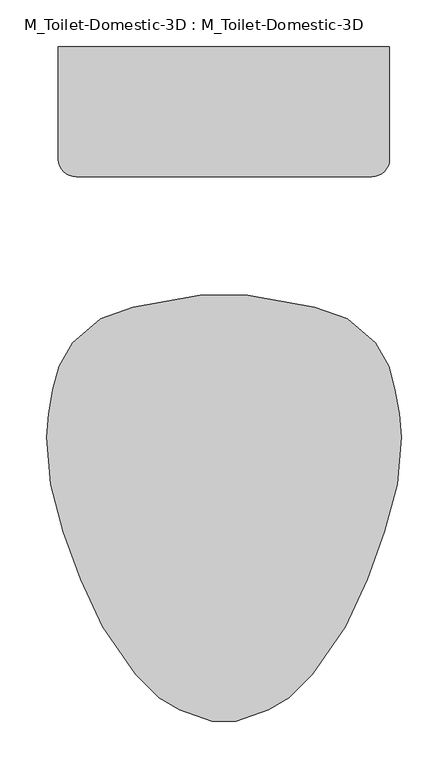
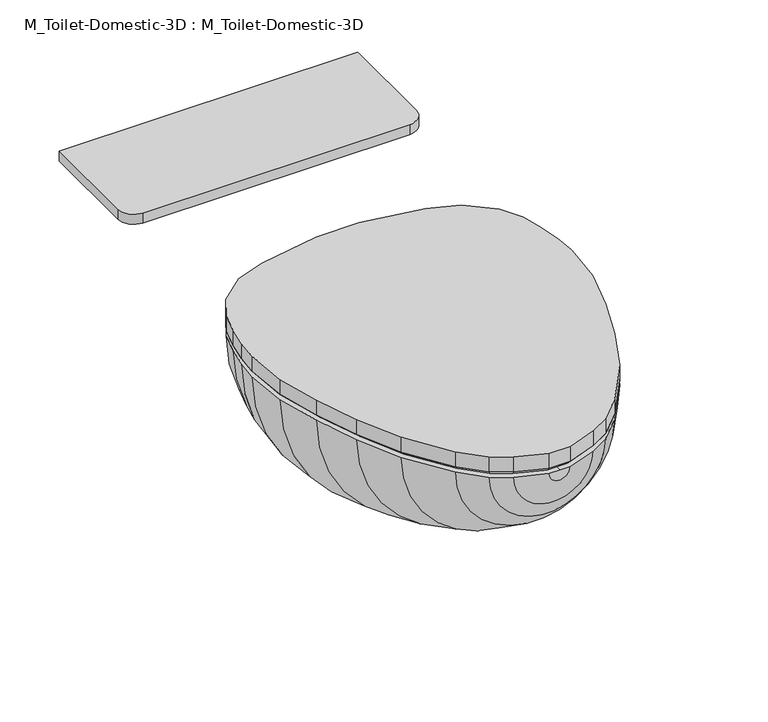
"""IFC4 building model written with IfcOpenShell, lengths in millimetres: flow terminal geometry, M_Toilet-Domestic-3D : M_Toilet-Domestic-3D."""

from ifc_helpers import new_model, si_unit, point, frame, frame_2d, origin, place, context, project, spatial, polyline, circle_curve, trimmed, segment, composite_curve, outline, extrude, faceted_brep, source, transform, mapped, element, save
from ifc_brep_helpers import plane_surface, revolved_surface, advanced_brep


def m_toilet_domestic_3d_m_toilet_domestic_3d_183bbd19(model_context):
    return source(origin(), model_context, "Body", "SolidModel", [
        advanced_brep(
        [(-25.4, 152.4, 361.95), (-97.4252791, 139.7, 361.95), (-132.3182423, 127.0, 361.95), (-162.5887836, 101.6, 361.95), (-176.9845865, 76.2, 361.95), (-183.790496, 50.8, 361.95), (-188.2862441, 25.3033453, 361.95), (-190.5, 0.0, 361.95), (-186.0724883, -50.6066907, 361.95), (-172.4088722, -101.6, 361.95), (-153.9191843, -152.4, 361.95), (-130.2307553, -203.2, 361.95), (-94.9900085, -254.0, 361.95), (-69.5900085, -279.4, 361.95), (-47.5929632, -292.1, 361.95), (-12.7, -304.8, 361.95), (0.0, -304.8, 361.95), (0.0, -284.592034, 361.95), (-12.5224565, -284.592034, 361.95), (-39.5113323, -274.7688865, 361.95), (-58.4178985, -263.8531754, 361.95), (-79.2146703, -243.0564036, 361.95), (-114.0255101, -192.8761202, 361.95), (-136.654021, -144.3491221, 361.95), (-154.575847, -95.1093097, 361.95), (-167.7238545, -46.0402777, 361.95), (-171.5645445, -2.1409906, 361.95), (-169.3087351, 23.6430284, 361.95), (-165.101298, 47.5045901, 361.95), (-159.5484355, 68.2281551, 361.95), (-146.1085923, 90.5605136, 361.95), (-121.9980886, 110.7916284, 361.95), (-94.1172813, 120.9394123, 361.95), (-22.0920022, 133.6394123, 361.95), (0.0, 133.6394123, 361.95), (0.0, 152.4, 361.95), (25.4, 152.4, 361.95), (22.0920022, 133.6394123, 361.95), (94.1172813, 120.9394123, 361.95), (121.9980886, 110.7916284, 361.95), (146.1085923, 90.5605136, 361.95), (159.5484355, 68.2281551, 361.95), (165.101298, 47.5045901, 361.95), (169.3087351, 23.6430284, 361.95), (171.5645445, -2.1409906, 361.95), (167.7238545, -46.0402777, 361.95), (154.575847, -95.1093097, 361.95), (136.654021, -144.3491221, 361.95), (114.0255101, -192.8761202, 361.95), (79.2146703, -243.0564036, 361.95), (58.4178985, -263.8531754, 361.95), (39.5113323, -274.7688865, 361.95), (12.5224565, -284.592034, 361.95), (12.7, -304.8, 361.95), (47.5929632, -292.1, 361.95), (69.5900085, -279.4, 361.95), (94.9900085, -254.0, 361.95), (130.2307553, -203.2, 361.95), (153.9191843, -152.4, 361.95), (172.4088722, -101.6, 361.95), (186.0724883, -50.6066907, 361.95), (190.5, 0.0, 361.95), (188.2862441, 25.3033453, 361.95), (183.790496, 50.8, 361.95), (176.9845865, 76.2, 361.95), (162.5887836, 101.6, 361.95), (132.3182423, 127.0, 361.95), (97.4252791, 139.7, 361.95)],
        [
            (0, 1),
            (1, 2),
            (2, 3),
            (3, 4),
            (4, 5),
            (5, 6),
            (6, 7),
            (7, 8),
            (8, 9),
            (9, 10),
            (10, 11),
            (11, 12),
            (12, 13),
            (13, 14),
            (14, 15),
            (15, 16),
            (16, 17),
            (17, 18),
            (18, 19),
            (19, 20),
            (20, 21),
            (21, 22),
            (22, 23),
            (23, 24),
            (24, 25),
            (25, 26),
            (26, 27),
            (27, 28),
            (28, 29),
            (29, 30),
            (30, 31),
            (31, 32),
            (32, 33),
            (33, 34),
            (34, 35),
            (35, 0),
            (36, 35),
            (34, 37),
            (37, 38),
            (38, 39),
            (39, 40),
            (40, 41),
            (41, 42),
            (42, 43),
            (43, 44),
            (44, 45),
            (45, 46),
            (46, 47),
            (47, 48),
            (48, 49),
            (49, 50),
            (50, 51),
            (51, 52),
            (52, 17),
            (16, 53),
            (53, 54),
            (54, 55),
            (55, 56),
            (56, 57),
            (57, 58),
            (58, 59),
            (59, 60),
            (60, 61),
            (61, 62),
            (62, 63),
            (63, 64),
            (64, 65),
            (65, 66),
            (66, 67),
            (67, 36),
            (67, 1, circle_curve(frame((0.0, 139.7, 361.95), z_axis=(0.0, 1.0, 0.0), x_axis=(-1.0, 0.0, 0.0)), 97.4252791)),
            (0, 36, circle_curve(frame((0.0, 152.4, 361.95), z_axis=(0.0, -1.0, 0.0), x_axis=(-1.0, 0.0, 0.0)), 25.4)),
            (66, 2, circle_curve(frame((0.0, 127.0, 361.95), z_axis=(0.0, 1.0, 0.0), x_axis=(-1.0, 0.0, 0.0)), 132.3182423)),
            (65, 3, circle_curve(frame((0.0, 101.6, 361.95), z_axis=(0.0, 1.0, 0.0), x_axis=(-1.0, 0.0, 0.0)), 162.5887836)),
            (64, 4, circle_curve(frame((0.0, 76.2, 361.95), z_axis=(0.0, 1.0, 0.0), x_axis=(-1.0, 0.0, 0.0)), 176.9845865)),
            (63, 5, circle_curve(frame((0.0, 50.8, 361.95), z_axis=(0.0, 1.0, 0.0), x_axis=(-1.0, 0.0, 0.0)), 183.790496)),
            (62, 6, circle_curve(frame((0.0, 25.3033453, 361.95), z_axis=(0.0, 1.0, 0.0), x_axis=(-1.0, 0.0, 0.0)), 188.2862441)),
            (61, 7, circle_curve(frame((0.0, 0.0, 361.95), z_axis=(0.0, 1.0, 0.0), x_axis=(-1.0, 0.0, 0.0)), 190.5)),
            (60, 8, circle_curve(frame((0.0, -50.6066907, 361.95), z_axis=(0.0, 1.0, 0.0), x_axis=(-1.0, 0.0, 0.0)), 186.0724883)),
            (59, 9, circle_curve(frame((0.0, -101.6, 361.95), z_axis=(0.0, 1.0, 0.0), x_axis=(-1.0, 0.0, 0.0)), 172.4088722)),
            (58, 10, circle_curve(frame((0.0, -152.4, 361.95), z_axis=(0.0, 1.0, 0.0), x_axis=(-1.0, 0.0, 0.0)), 153.9191843)),
            (57, 11, circle_curve(frame((0.0, -203.2, 361.95), z_axis=(0.0, 1.0, 0.0), x_axis=(-1.0, 0.0, 0.0)), 130.2307553)),
            (56, 12, circle_curve(frame((0.0, -254.0, 361.95), z_axis=(0.0, 1.0, 0.0), x_axis=(-1.0, 0.0, 0.0)), 94.9900085)),
            (55, 13, circle_curve(frame((0.0, -279.4, 361.95), z_axis=(0.0, 1.0, 0.0), x_axis=(-1.0, 0.0, 0.0)), 69.5900085)),
            (54, 14, circle_curve(frame((0.0, -292.1, 361.95), z_axis=(0.0, 1.0, 0.0), x_axis=(-1.0, 0.0, 0.0)), 47.5929632)),
            (53, 15, circle_curve(frame((0.0, -304.8, 361.95), z_axis=(0.0, 1.0, 0.0), x_axis=(-1.0, 0.0, 0.0)), 12.7)),
            (52, 18, circle_curve(frame((0.0, -284.592034, 361.95), z_axis=(0.0, 1.0, 0.0), x_axis=(-1.0, 0.0, 0.0)), 12.5224565)),
            (51, 19, circle_curve(frame((0.0, -274.7688865, 361.95), z_axis=(0.0, 1.0, 0.0), x_axis=(-1.0, 0.0, 0.0)), 39.5113323)),
            (50, 20, circle_curve(frame((0.0, -263.8531754, 361.95), z_axis=(0.0, 1.0, 0.0), x_axis=(-1.0, 0.0, 0.0)), 58.4178985)),
            (49, 21, circle_curve(frame((0.0, -243.0564036, 361.95), z_axis=(0.0, 1.0, 0.0), x_axis=(-1.0, 0.0, 0.0)), 79.2146703)),
            (48, 22, circle_curve(frame((0.0, -192.8761202, 361.95), z_axis=(0.0, 1.0, 0.0), x_axis=(-1.0, 0.0, 0.0)), 114.0255101)),
            (47, 23, circle_curve(frame((0.0, -144.3491221, 361.95), z_axis=(0.0, 1.0, 0.0), x_axis=(-1.0, 0.0, 0.0)), 136.654021)),
            (46, 24, circle_curve(frame((0.0, -95.1093097, 361.95), z_axis=(0.0, 1.0, 0.0), x_axis=(-1.0, 0.0, 0.0)), 154.575847)),
            (45, 25, circle_curve(frame((0.0, -46.0402777, 361.95), z_axis=(0.0, 1.0, 0.0), x_axis=(-1.0, 0.0, 0.0)), 167.7238545)),
            (44, 26, circle_curve(frame((0.0, -2.1409906, 361.95), z_axis=(0.0, 1.0, 0.0), x_axis=(-1.0, 0.0, 0.0)), 171.5645445)),
            (43, 27, circle_curve(frame((0.0, 23.6430284, 361.95), z_axis=(0.0, 1.0, 0.0), x_axis=(-1.0, 0.0, 0.0)), 169.3087351)),
            (42, 28, circle_curve(frame((0.0, 47.5045901, 361.95), z_axis=(0.0, 1.0, 0.0), x_axis=(-1.0, 0.0, 0.0)), 165.101298)),
            (41, 29, circle_curve(frame((0.0, 68.2281551, 361.95), z_axis=(0.0, 1.0, 0.0), x_axis=(-1.0, 0.0, 0.0)), 159.5484355)),
            (40, 30, circle_curve(frame((0.0, 90.5605136, 361.95), z_axis=(0.0, 1.0, 0.0), x_axis=(-1.0, 0.0, 0.0)), 146.1085923)),
            (39, 31, circle_curve(frame((0.0, 110.7916284, 361.95), z_axis=(0.0, 1.0, 0.0), x_axis=(-1.0, 0.0, 0.0)), 121.9980886)),
            (38, 32, circle_curve(frame((0.0, 120.9394123, 361.95), z_axis=(0.0, 1.0, 0.0), x_axis=(-1.0, 0.0, 0.0)), 94.1172813)),
            (37, 33, circle_curve(frame((0.0, 133.6394123, 361.95), z_axis=(0.0, 1.0, 0.0), x_axis=(-1.0, 0.0, 0.0)), 22.0920022)),
        ],
        [
            plane_surface(frame((0.0, 175.1599017, 361.95), z_axis=(0.0, 0.0, 1.0), x_axis=(-1.0, 0.0, 0.0))),
            plane_surface(frame((0.0, 175.1599017, 361.95), z_axis=(0.0, 0.0, 1.0), x_axis=(1.0, 0.0, 0.0))),
            revolved_surface(polyline([(-25.4, 152.4, 361.95), (-97.4252791, 139.7, 361.95)]), (0.0, 175.1599017, 361.95), (0.0, -1.0, 0.0)),
            revolved_surface(polyline([(-97.4252791, 139.7, 361.95), (-132.3182423, 127.0, 361.95)]), (0.0, 175.1599017, 361.95), (0.0, -1.0, 0.0)),
            revolved_surface(polyline([(-132.3182423, 127.0, 361.95), (-162.5887836, 101.6, 361.95)]), (0.0, 175.1599017, 361.95), (0.0, -1.0, 0.0)),
            revolved_surface(polyline([(-162.5887836, 101.6, 361.95), (-176.9845865, 76.2, 361.95)]), (0.0, 175.1599017, 361.95), (0.0, -1.0, 0.0)),
            revolved_surface(polyline([(-176.9845865, 76.2, 361.95), (-183.790496, 50.8, 361.95)]), (0.0, 175.1599017, 361.95), (0.0, -1.0, 0.0)),
            revolved_surface(polyline([(-183.790496, 50.8, 361.95), (-188.2862441, 25.3033453, 361.95)]), (0.0, 175.1599017, 361.95), (0.0, -1.0, 0.0)),
            revolved_surface(polyline([(-188.2862441, 25.3033453, 361.95), (-190.5, 0.0, 361.95)]), (0.0, 175.1599017, 361.95), (0.0, -1.0, 0.0)),
            revolved_surface(polyline([(-190.5, 0.0, 361.95), (-186.0724883, -50.6066907, 361.95)]), (0.0, 175.1599017, 361.95), (0.0, -1.0, 0.0)),
            revolved_surface(polyline([(-186.0724883, -50.6066907, 361.95), (-172.4088722, -101.6, 361.95)]), (0.0, 175.1599017, 361.95), (0.0, -1.0, 0.0)),
            revolved_surface(polyline([(-172.4088722, -101.6, 361.95), (-153.9191843, -152.4, 361.95)]), (0.0, 175.1599017, 361.95), (0.0, -1.0, 0.0)),
            revolved_surface(polyline([(-153.9191843, -152.4, 361.95), (-130.2307553, -203.2, 361.95)]), (0.0, 175.1599017, 361.95), (0.0, -1.0, 0.0)),
            revolved_surface(polyline([(-130.2307553, -203.2, 361.95), (-94.9900085, -254.0, 361.95)]), (0.0, 175.1599017, 361.95), (0.0, -1.0, 0.0)),
            revolved_surface(polyline([(-94.9900085, -254.0, 361.95), (-69.5900085, -279.4, 361.95)]), (0.0, 175.1599017, 361.95), (0.0, -1.0, 0.0)),
            revolved_surface(polyline([(-69.5900085, -279.4, 361.95), (-47.5929632, -292.1, 361.95)]), (0.0, 175.1599017, 361.95), (0.0, -1.0, 0.0)),
            revolved_surface(polyline([(-47.5929632, -292.1, 361.95), (-12.7, -304.8, 361.95)]), (0.0, 175.1599017, 361.95), (0.0, -1.0, 0.0)),
            plane_surface(frame((0.0, -304.8, 361.95), z_axis=(0.0, -1.0, 0.0), x_axis=(-1.0, 0.0, 0.0))),
            plane_surface(frame((0.0, -284.592034, 361.95), z_axis=(0.0, 1.0, 0.0), x_axis=(-1.0, 0.0, 0.0))),
            revolved_surface(polyline([(-12.5224565, -284.592034, 361.95), (-39.5113323, -274.7688865, 361.95)]), (0.0, 175.1599017, 361.95), (0.0, -1.0, 0.0)),
            revolved_surface(polyline([(-39.5113323, -274.7688865, 361.95), (-58.4178985, -263.8531754, 361.95)]), (0.0, 175.1599017, 361.95), (0.0, -1.0, 0.0)),
            revolved_surface(polyline([(-58.4178985, -263.8531754, 361.95), (-79.2146703, -243.0564036, 361.95)]), (0.0, 175.1599017, 361.95), (0.0, -1.0, 0.0)),
            revolved_surface(polyline([(-79.2146703, -243.0564036, 361.95), (-114.0255101, -192.8761202, 361.95)]), (0.0, 175.1599017, 361.95), (0.0, -1.0, 0.0)),
            revolved_surface(polyline([(-114.0255101, -192.8761202, 361.95), (-136.654021, -144.3491221, 361.95)]), (0.0, 175.1599017, 361.95), (0.0, -1.0, 0.0)),
            revolved_surface(polyline([(-136.654021, -144.3491221, 361.95), (-154.575847, -95.1093097, 361.95)]), (0.0, 175.1599017, 361.95), (0.0, -1.0, 0.0)),
            revolved_surface(polyline([(-154.575847, -95.1093097, 361.95), (-167.7238545, -46.0402777, 361.95)]), (0.0, 175.1599017, 361.95), (0.0, -1.0, 0.0)),
            revolved_surface(polyline([(-167.7238545, -46.0402777, 361.95), (-171.5645445, -2.1409906, 361.95)]), (0.0, 175.1599017, 361.95), (0.0, -1.0, 0.0)),
            revolved_surface(polyline([(-171.5645445, -2.1409906, 361.95), (-169.3087351, 23.6430284, 361.95)]), (0.0, 175.1599017, 361.95), (0.0, -1.0, 0.0)),
            revolved_surface(polyline([(-169.3087351, 23.6430284, 361.95), (-165.101298, 47.5045901, 361.95)]), (0.0, 175.1599017, 361.95), (0.0, -1.0, 0.0)),
            revolved_surface(polyline([(-165.101298, 47.5045901, 361.95), (-159.5484355, 68.2281551, 361.95)]), (0.0, 175.1599017, 361.95), (0.0, -1.0, 0.0)),
            revolved_surface(polyline([(-159.5484355, 68.2281551, 361.95), (-146.1085923, 90.5605136, 361.95)]), (0.0, 175.1599017, 361.95), (0.0, -1.0, 0.0)),
            revolved_surface(polyline([(-146.1085923, 90.5605136, 361.95), (-121.9980886, 110.7916284, 361.95)]), (0.0, 175.1599017, 361.95), (0.0, -1.0, 0.0)),
            revolved_surface(polyline([(-121.9980886, 110.7916284, 361.95), (-94.1172813, 120.9394123, 361.95)]), (0.0, 175.1599017, 361.95), (0.0, -1.0, 0.0)),
            revolved_surface(polyline([(-94.1172813, 120.9394123, 361.95), (-22.0920022, 133.6394123, 361.95)]), (0.0, 175.1599017, 361.95), (0.0, -1.0, 0.0)),
            plane_surface(frame((0.0, 133.6394123, 361.95), z_axis=(0.0, -1.0, 0.0), x_axis=(-1.0, 0.0, 0.0))),
            plane_surface(frame((0.0, 152.4, 361.95), z_axis=(0.0, 1.0, 0.0), x_axis=(-1.0, 0.0, 0.0))),
        ],
        [
            (0, [[1, 2, 3, 4, 5, 6, 7, 8, 9, 10, 11, 12, 13, 14, 15, 16, 17, 18, 19, 20, 21, 22, 23, 24, 25, 26, 27, 28, 29, 30, 31, 32, 33, 34, 35, 36]]),
            (1, [[37, -35, 38, 39, 40, 41, 42, 43, 44, 45, 46, 47, 48, 49, 50, 51, 52, 53, 54, -17, 55, 56, 57, 58, 59, 60, 61, 62, 63, 64, 65, 66, 67, 68, 69, 70]]),
            (2, [[71, -1, 72, -70]]),
            (3, [[73, -2, -71, -69]]),
            (4, [[74, -3, -73, -68]]),
            (5, [[75, -4, -74, -67]]),
            (6, [[76, -5, -75, -66]]),
            (7, [[77, -6, -76, -65]]),
            (8, [[78, -7, -77, -64]]),
            (9, [[79, -8, -78, -63]]),
            (10, [[80, -9, -79, -62]]),
            (11, [[81, -10, -80, -61]]),
            (12, [[82, -11, -81, -60]]),
            (13, [[83, -12, -82, -59]]),
            (14, [[84, -13, -83, -58]]),
            (15, [[85, -14, -84, -57]]),
            (16, [[86, -15, -85, -56]]),
            (17, [[-16, -86, -55]]),
            (18, [[87, -18, -54]]),
            (19, [[88, -19, -87, -53]]),
            (20, [[89, -20, -88, -52]]),
            (21, [[90, -21, -89, -51]]),
            (22, [[91, -22, -90, -50]]),
            (23, [[92, -23, -91, -49]]),
            (24, [[93, -24, -92, -48]]),
            (25, [[94, -25, -93, -47]]),
            (26, [[95, -26, -94, -46]]),
            (27, [[96, -27, -95, -45]]),
            (28, [[97, -28, -96, -44]]),
            (29, [[98, -29, -97, -43]]),
            (30, [[99, -30, -98, -42]]),
            (31, [[100, -31, -99, -41]]),
            (32, [[101, -32, -100, -40]]),
            (33, [[102, -33, -101, -39]]),
            (34, [[-34, -102, -38]]),
            (35, [[-72, -36, -37]]),
        ],
    ),
        faceted_brep([(-97.4252791, 139.7, 368.3), (-132.3182423, 127.0, 368.3), (-162.5887836, 101.6, 368.3), (-176.9845865, 76.2, 368.3), (-183.790496, 50.8, 368.3), (-188.2862441, 25.3033453, 368.3), (-190.5, 0.0, 368.3), (-186.0724883, -50.6066907, 368.3), (-172.4088722, -101.6, 368.3), (-153.9191843, -152.4, 368.3), (-130.2307553, -203.2, 368.3), (-94.9900085, -254.0, 368.3), (-69.5900085, -279.4, 368.3), (-47.5929632, -292.1, 368.3), (-12.7, -304.8, 368.3), (12.7, -304.8, 368.3), (47.5929632, -292.1, 368.3), (69.5900085, -279.4, 368.3), (94.9900085, -254.0, 368.3), (130.2307553, -203.2, 368.3), (153.9191843, -152.4, 368.3), (172.4088722, -101.6, 368.3), (186.0724883, -50.6066907, 368.3), (190.5, 0.0, 368.3), (188.2862441, 25.3033453, 368.3), (183.790496, 50.8, 368.3), (176.9845865, 76.2, 368.3), (162.5887836, 101.6, 368.3), (132.3182423, 127.0, 368.3), (97.4252791, 139.7, 368.3), (25.4, 152.4, 368.3), (-25.4, 152.4, 368.3), (-95.7755003, 133.5429415, 361.95), (-24.844447, 146.05, 361.95), (24.844447, 146.05, 361.95), (95.7755003, 133.5429415, 361.95), (129.0942628, 121.4159037, 361.95), (157.6293435, 97.472128, 361.95), (171.060664, 73.773864, 361.95), (177.5851102, 49.4242991, 361.95), (181.9845715, 24.4737144, 361.95), (184.125744, 0.0, 361.95), (179.7950716, -49.4998127, 361.95), (166.347, -99.688699, 361.95), (148.0469602, -149.9676451, 361.95), (124.7045808, -200.0255393, 361.95), (90.0971582, -249.9125941, 361.95), (65.691017, -274.3187354, 361.95), (44.8990862, -286.3229622, 361.95), (11.5803237, -298.45, 361.95), (-11.5803237, -298.45, 361.95), (-44.8990862, -286.3229622, 361.95), (-65.691017, -274.3187354, 361.95), (-90.0971582, -249.9125941, 361.95), (-124.7045808, -200.0255393, 361.95), (-148.0469602, -149.9676451, 361.95), (-166.347, -99.688699, 361.95), (-179.7950716, -49.4998127, 361.95), (-184.125744, 0.0, 361.95), (-181.9845715, 24.4737144, 361.95), (-177.5851102, 49.4242991, 361.95), (-171.060664, 73.773864, 361.95), (-157.6293435, 97.472128, 361.95), (-129.0942628, 121.4159037, 361.95)], [[[0, 1, 2, 3, 4, 5, 6, 7, 8, 9, 10, 11, 12, 13, 14, 15, 16, 17, 18, 19, 20, 21, 22, 23, 24, 25, 26, 27, 28, 29, 30, 31]], [[32, 33, 34, 35, 36, 37, 38, 39, 40, 41, 42, 43, 44, 45, 46, 47, 48, 49, 50, 51, 52, 53, 54, 55, 56, 57, 58, 59, 60, 61, 62, 63]], [[32, 63, 1, 0]], [[63, 62, 2, 1]], [[62, 61, 3, 2]], [[61, 60, 4, 3]], [[60, 59, 5, 4]], [[59, 58, 6, 5]], [[58, 57, 7, 6]], [[57, 56, 8, 7]], [[56, 55, 9, 8]], [[55, 54, 10, 9]], [[54, 53, 11, 10]], [[53, 52, 12, 11]], [[52, 51, 13, 12]], [[51, 50, 14, 13]], [[50, 49, 15, 14]], [[49, 48, 16, 15]], [[48, 47, 17, 16]], [[47, 46, 18, 17]], [[46, 45, 19, 18]], [[45, 44, 20, 19]], [[44, 43, 21, 20]], [[43, 42, 22, 21]], [[42, 41, 23, 22]], [[41, 40, 24, 23]], [[40, 39, 25, 24]], [[39, 38, 26, 25]], [[38, 37, 27, 26]], [[37, 36, 28, 27]], [[36, 35, 29, 28]], [[35, 34, 30, 29]], [[34, 33, 31, 30]], [[33, 32, 0, 31]]]),
        extrude(outline(composite_curve([segment(polyline([(177.8, 419.1), (177.8, 298.45)]), True, "CONTINUOUS"), segment(trimmed(circle_curve(frame_2d((158.75, 298.45)), 19.05), [point((177.8, 298.45))], [point((158.75, 279.4))], False, "CARTESIAN"), True, "CONTINUOUS"), segment(polyline([(158.75, 279.4), (-158.75, 279.4)]), True, "CONTINUOUS"), segment(trimmed(circle_curve(frame_2d((-158.75, 298.45)), 19.05), [point((-158.75, 279.4))], [point((-177.8, 298.45))], False, "CARTESIAN"), True, "CONTINUOUS"), segment(polyline([(-177.8, 298.45), (-177.8, 419.1), (177.8, 419.1)]), True, "CONTINUOUS")], self_intersect=False)), frame((0.0, 0.0, 374.65), z_axis=(0.0, 0.0, 1.0), x_axis=(1.0, 0.0, 0.0)), (0.0, 0.0, 1.0), 12.5681453),
        extrude(outline(polyline([(-162.5887836, 101.6), (-132.3182423, 127.0), (-97.4252791, 139.7), (-25.4, 152.4), (25.4, 152.4), (97.4252791, 139.7), (132.3182423, 127.0), (162.5887836, 101.6), (176.9845865, 76.2), (183.790496, 50.8), (188.2862441, 25.3033453), (190.5, 0.0), (186.0724883, -50.6066907), (172.4088722, -101.6), (153.9191843, -152.4), (130.2307553, -203.2), (94.9900085, -254.0), (69.5900085, -279.4), (47.5929632, -292.1), (12.7, -304.8), (-12.7, -304.8), (-47.5929632, -292.1), (-69.5900085, -279.4), (-94.9900085, -254.0), (-130.2307553, -203.2), (-153.9191843, -152.4), (-172.4088722, -101.6), (-186.0724883, -50.6066907), (-190.5, 0.0), (-188.2862441, 25.3033453), (-183.790496, 50.8), (-176.9845865, 76.2), (-162.5887836, 101.6)])), frame((0.0, 0.0, 368.3), z_axis=(0.0, 0.0, 1.0), x_axis=(1.0, 0.0, 0.0)), (0.0, 0.0, 1.0), 19.05),
    ])


if __name__ == "__main__":
    model = new_model("IFC4")
    model_context = context("Model", 3, world=origin())
    ifc_project = project(units=[si_unit("LENGTHUNIT", "METRE", prefix="MILLI")], contexts=[model_context])
    site = spatial("IfcSite", under=ifc_project)
    building = spatial("IfcBuilding", under=site)
    placement = place(None, origin())
    m_toilet_domestic_3d_m_toilet_domestic_3d_shape = m_toilet_domestic_3d_m_toilet_domestic_3d_183bbd19(model_context)
    element("IfcFlowTerminal", 1, ObjectType="M_Toilet-Domestic-3D : M_Toilet-Domestic-3D", at=placement, inside=building, context=model_context, shape_type="MappedRepresentation", body=[
        mapped(m_toilet_domestic_3d_m_toilet_domestic_3d_shape, transform((0.0, 0.0, 0.0), x_axis=(1.0, 0.0, 0.0), y_axis=(0.0, 1.0, 0.0), z_axis=(0.0, 0.0, 1.0))),
    ])
    save(model, "model.ifc")

# Revit data of these elements
# Type "M_Toilet-Domestic-3D : M_Toilet-Domestic-3D"
#   Bowl/Basin Material = Porcelain, Linen
#   Seat Material = Laminate, Linen, Matte
#   Default Elevation = 0
# Element 1 (IfcFlowTerminal, "M_Toilet-Domestic-3D : M_Toilet-Domestic-3D")
#   Materials on its faces: "Porcelain, Linen", "Laminate, Linen, Matte"
# Materials
#   "Porcelain, Linen": class "Ceramic", colour RGB 249 239 230, transparency 0, Description = "Porcelain, linen", Cost = 0
#   "Laminate, Linen, Matte": class "Plastic", colour RGB 249 239 230, transparency 0, Description = "Plastic Laminate - Linen, Matte", Cost = 0
